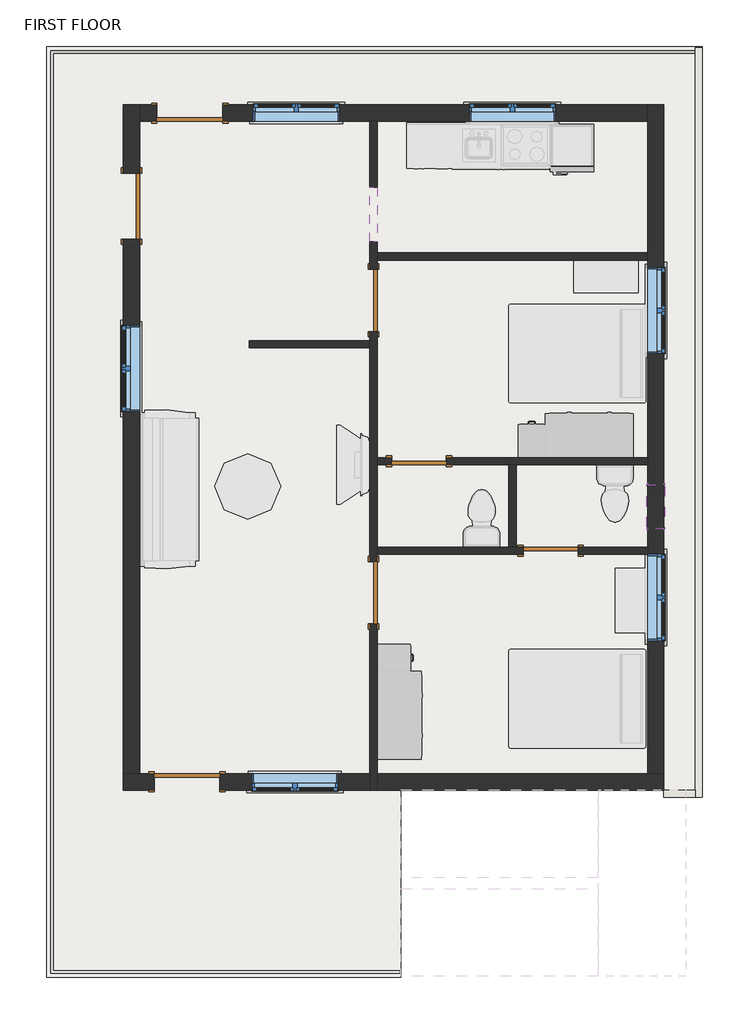
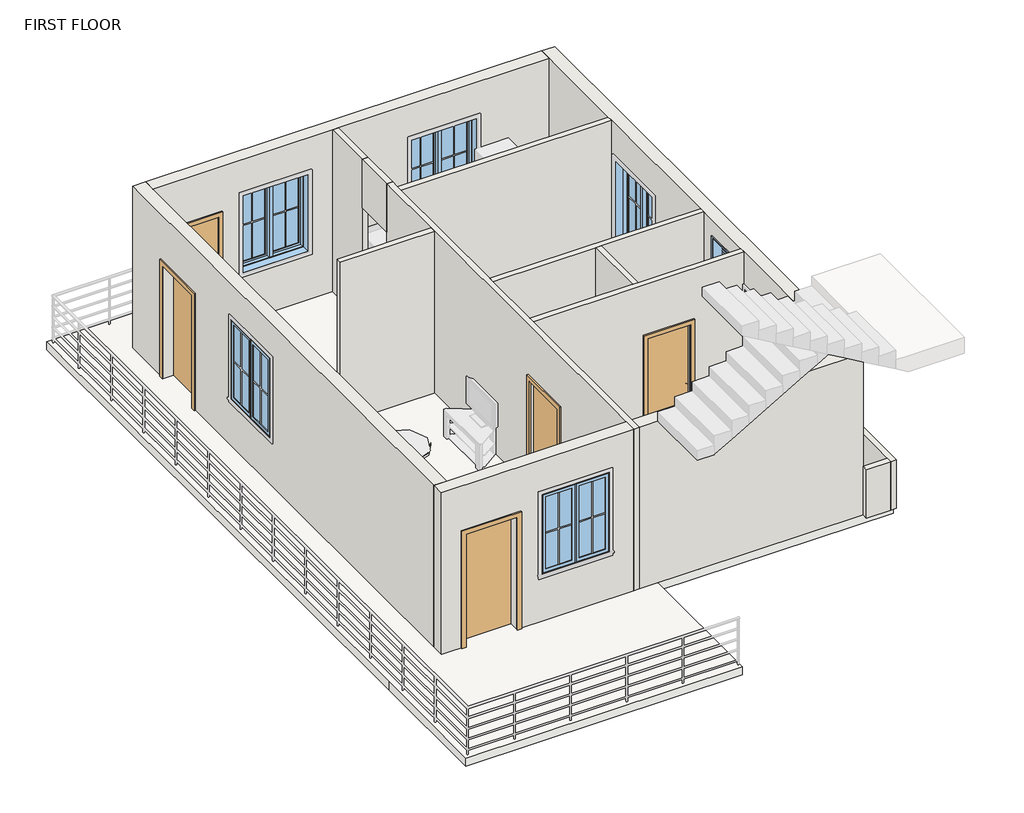
# One storey, part 1 of 3: 15 walls, 7 doors, 7 windows, 1 slab.
"""IFC4 building model written with IfcOpenShell, lengths in millimetres."""

from ifc_helpers import new_model, si_unit, frame, origin, place, context, project, spatial, polyline, outline, extrude, faceted_brep, transform, mapped, element, save
from components import m_single_flush_0762_x_2032mm_63ada305, m_single_flush_0762_x_2032mm_debabc81, m_single_flush_0864_x_2032mm_c62421c0, m_single_flush_0915_x_2134mm_43602619, m_single_flush_0915_x_2134mm_1ddf3370, m_window_casement_double_1200_x_1500mm_04159c99, window_f2d8fef0

model = new_model("IFC4")

# Units and contexts
model_context = context("Model", 3, world=origin())
ifc_project = project(units=[si_unit("LENGTHUNIT", "METRE", prefix="MILLI")], contexts=[model_context])

# Site, building, storey
site = spatial("IfcSite", under=ifc_project)
building = spatial("IfcBuilding", under=site)
storey = spatial("IfcBuildingStorey", under=building, Name="FIRST FLOOR", Elevation=3200.4)

# Doors
placement = place(None, origin())
m_single_flush_0762_x_2032mm_shape = m_single_flush_0762_x_2032mm_63ada305(model_context)
element("IfcDoor", 1, ObjectType="M_Single-Flush : 0762 x 2032mm", at=placement, inside=storey, context=model_context, shape_type="MappedRepresentation", body=[
    mapped(m_single_flush_0762_x_2032mm_shape, transform((2297.1455952, -1088.4648653, 3200.4), x_axis=(-1.0, 0.0, 0.0), y_axis=(0.0, -1.0, 0.0), z_axis=(0.0, 0.0, 1.0))),
])
m_single_flush_0762_x_2032mm_2_shape = m_single_flush_0762_x_2032mm_debabc81(model_context)
element("IfcDoor", 2, ObjectType="M_Single-Flush : 0762 x 2032mm", at=placement, inside=storey, context=model_context, shape_type="MappedRepresentation", body=[
    mapped(m_single_flush_0762_x_2032mm_2_shape, transform((466.7455952, 156.1351347, 3200.4), x_axis=(-1.0, 0.0, 0.0), y_axis=(0.0, -1.0, 0.0), z_axis=(0.0, 0.0, 1.0))),
])
m_single_flush_0864_x_2032mm_shape = m_single_flush_0864_x_2032mm_c62421c0(model_context)
element("IfcDoor", 3, ObjectType="M_Single-Flush : 0864 x 2032mm", at=placement, inside=storey, context=model_context, shape_type="MappedRepresentation", body=[
    mapped(m_single_flush_0864_x_2032mm_shape, transform((-165.0544048, 2391.3351347, 3200.4), x_axis=(0.0, 1.0, 0.0), y_axis=(-1.0, 0.0, 0.0), z_axis=(0.0, 0.0, 1.0))),
])
element("IfcDoor", 4, ObjectType="M_Single-Flush : 0864 x 2032mm", at=placement, inside=storey, context=model_context, shape_type="MappedRepresentation", body=[
    mapped(m_single_flush_0864_x_2032mm_shape, transform((-165.0544048, -1671.2648653, 3200.4), x_axis=(0.0, 1.0, 0.0), y_axis=(-1.0, 0.0, 0.0), z_axis=(0.0, 0.0, 1.0))),
])
m_single_flush_0915_x_2134mm_shape = m_single_flush_0915_x_2134mm_43602619(model_context)
element("IfcDoor", 5, ObjectType="M_Single-Flush : 0915 x 2134mm", at=placement, inside=storey, context=model_context, shape_type="MappedRepresentation", body=[
    mapped(m_single_flush_0915_x_2134mm_shape, transform((-3530.5544048, 3703.0351347, 3200.4), x_axis=(0.0, 1.0, 0.0), y_axis=(-1.0, 0.0, 0.0), z_axis=(0.0, 0.0, 1.0))),
])
element("IfcDoor", 6, ObjectType="M_Single-Flush : 0915 x 2134mm", at=placement, inside=storey, context=model_context, shape_type="MappedRepresentation", body=[
    mapped(m_single_flush_0915_x_2134mm_shape, transform((-2758.7544048, -4301.5648653, 3200.4), x_axis=(-1.0, 0.0, 0.0), y_axis=(0.0, -1.0, 0.0), z_axis=(0.0, 0.0, 1.0))),
])
m_single_flush_0915_x_2134mm_2_shape = m_single_flush_0915_x_2134mm_1ddf3370(model_context)
element("IfcDoor", 7, ObjectType="M_Single-Flush : 0915 x 2134mm", at=placement, inside=storey, context=model_context, shape_type="MappedRepresentation", body=[
    mapped(m_single_flush_0915_x_2134mm_2_shape, transform((-2718.7544048, 4994.8351347, 3200.4), x_axis=(-1.0, 0.0, 0.0), y_axis=(0.0, -1.0, 0.0), z_axis=(0.0, 0.0, 1.0))),
])

# Slab
element("IfcSlab", 8, ObjectType="6\" floor", at=placement, inside=storey, context=model_context, shape_type="SweptSolid", body=[
    extrude(outline(polyline([(4406.9455952, 5921.9351347), (4406.9455952, -4415.8648653), (215.9455952, -4415.8648653), (215.9455952, -7021.8741001), (-4711.6544048, -7021.8741001), (-4711.6544048, -4637.8294487), (-4711.6544048, 5921.9351347), (4406.9455952, 5921.9351347)])), frame((0.0, 0.0, 3048.0), z_axis=(0.0, 0.0, 1.0), x_axis=(1.0, 0.0, 0.0)), (0.0, 0.0, 1.0), 152.4),
])

# Walls
element("IfcWall", 9, ObjectType="4\" wall", at=placement, inside=storey, context=model_context, shape_type="Brep", body=[
    faceted_brep([(-215.8544048, 3204.1351347, 3200.4), (-215.8544048, 2823.3351347, 3200.4), (-215.8544048, 2823.3351347, 5232.4), (-215.8544048, 1959.3351347, 5232.4), (-215.8544048, 1959.3351347, 3200.4), (-215.8544048, 1832.5351347, 3200.4), (-215.8544048, 1730.9351347, 3200.4), (-215.8544048, -1239.2648653, 3200.4), (-215.8544048, -1239.2648653, 5232.4), (-215.8544048, -2103.2648653, 5232.4), (-215.8544048, -2103.2648653, 3200.4), (-215.8544048, -4187.2648653, 3200.4), (-215.8544048, -4415.8648653, 3200.4), (-215.8544048, -4415.8648653, 6248.4), (-215.8544048, -4187.2648653, 6248.4), (-215.8544048, 1730.9351347, 6248.4), (-215.8544048, 1832.5351347, 6248.4), (-215.8544048, 3204.1351347, 6248.4), (-215.8544048, 3204.1351347, 5334.0), (-114.2544048, 2823.3351347, 5232.4), (-114.2544048, 2823.3351347, 3200.4), (-114.2544048, 2950.1351347, 3200.4), (-114.2544048, 3051.7351347, 3200.4), (-114.2544048, 3204.1351347, 3200.4), (-114.2544048, 3204.1351347, 5334.0), (-114.2544048, 3204.1351347, 6248.4), (-114.2544048, 3051.7351347, 6248.4), (-114.2544048, 2950.1351347, 6248.4), (-114.2544048, 206.9351347, 6248.4), (-114.2544048, 105.3351347, 6248.4), (-114.2544048, -1037.6648653, 6248.4), (-114.2544048, -1139.2648653, 6248.4), (-114.2544048, -4187.2648653, 6248.4), (-114.2544048, -4415.8648653, 6248.4), (-114.2544048, -4415.8648653, 3200.4), (-114.2544048, -4187.2648653, 3200.4), (-114.2544048, -2103.2648653, 3200.4), (-114.2544048, -2103.2648653, 5232.4), (-114.2544048, -1239.2648653, 5232.4), (-114.2544048, -1239.2648653, 3200.4), (-114.2544048, -1139.2648653, 3200.4), (-114.2544048, -1037.6648653, 3200.4), (-114.2544048, 105.3351347, 3200.4), (-114.2544048, 206.9351347, 3200.4), (-114.2544048, 1959.3351347, 3200.4), (-114.2544048, 1959.3351347, 5232.4)], [[[0, 1, 2, 3, 4, 5, 6, 7, 8, 9, 10, 11, 12, 13, 14, 15, 16, 17, 18]], [[19, 20, 21, 22, 23, 24, 25, 26, 27, 28, 29, 30, 31, 32, 33, 34, 35, 36, 37, 38, 39, 40, 41, 42, 43, 44, 45]], [[34, 12, 11, 10, 36, 35]], [[23, 22, 21, 20, 1, 0]], [[44, 43, 42, 41, 40, 39, 7, 6, 5, 4]], [[17, 16, 15, 14, 13, 33, 32, 31, 30, 29, 28, 27, 26, 25]], [[0, 18, 17, 25, 24, 23]], [[13, 12, 34, 33]], [[8, 38, 37, 9]], [[9, 37, 36, 10]], [[4, 3, 45, 44]], [[3, 2, 19, 45]], [[2, 1, 20, 19]], [[38, 8, 7, 39]]]),
])
element("IfcWall", 10, ObjectType="4\" wall", at=placement, inside=storey, context=model_context, shape_type="Brep", body=[
    faceted_brep([(-114.2544048, -1139.2648653, 3200.4), (1916.1455952, -1139.2648653, 3200.4), (1916.1455952, -1139.2648653, 5232.4), (2678.1455952, -1139.2648653, 5232.4), (2678.1455952, -1139.2648653, 3200.4), (3644.9455952, -1139.2648653, 3200.4), (3644.9455952, -1139.2648653, 4100.4), (3644.9455952, -1139.2648653, 5600.4), (3644.9455952, -1139.2648653, 6248.4), (-114.2544048, -1139.2648653, 6248.4), (1916.1455952, -1037.6648653, 5232.4), (1916.1455952, -1037.6648653, 3200.4), (1816.1455952, -1037.6648653, 3200.4), (1714.5455952, -1037.6648653, 3200.4), (-114.2544048, -1037.6648653, 3200.4), (-114.2544048, -1037.6648653, 6248.4), (1714.5455952, -1037.6648653, 6248.4), (1816.1455952, -1037.6648653, 6248.4), (3644.9455952, -1037.6648653, 6248.4), (3644.9455952, -1037.6648653, 3200.4), (2678.1455952, -1037.6648653, 3200.4), (2678.1455952, -1037.6648653, 5232.4)], [[[0, 1, 2, 3, 4, 5, 6, 7, 8, 9]], [[10, 11, 12, 13, 14, 15, 16, 17, 18, 19, 20, 21]], [[20, 19, 5, 4]], [[14, 13, 12, 11, 1, 0]], [[9, 8, 18, 17, 16, 15]], [[8, 7, 6, 5, 19, 18]], [[0, 9, 15, 14]], [[2, 1, 11, 10]], [[3, 2, 10, 21]], [[4, 3, 21, 20]]]),
])
element("IfcWall", 11, ObjectType="4\" wall", at=placement, inside=storey, context=model_context, shape_type="Brep", body=[
    faceted_brep([(85.7455952, 206.9351347, 5232.4), (85.7455952, 206.9351347, 3200.4), (-114.2544048, 206.9351347, 3200.4), (-114.2544048, 206.9351347, 6248.4), (3644.9455952, 206.9351347, 6248.4), (3644.9455952, 206.9351347, 3200.4), (847.7455952, 206.9351347, 3200.4), (847.7455952, 206.9351347, 5232.4), (-114.2544048, 105.3351347, 3200.4), (85.7455952, 105.3351347, 3200.4), (85.7455952, 105.3351347, 5232.4), (847.7455952, 105.3351347, 5232.4), (847.7455952, 105.3351347, 3200.4), (1714.5455952, 105.3351347, 3200.4), (1816.1455952, 105.3351347, 3200.4), (3644.9455952, 105.3351347, 3200.4), (3644.9455952, 105.3351347, 6248.4), (1816.1455952, 105.3351347, 6248.4), (1714.5455952, 105.3351347, 6248.4), (-114.2544048, 105.3351347, 6248.4)], [[[0, 1, 2, 3, 4, 5, 6, 7]], [[8, 9, 10, 11, 12, 13, 14, 15, 16, 17, 18, 19]], [[6, 5, 15, 14, 13, 12]], [[2, 1, 9, 8]], [[4, 3, 19, 18, 17, 16]], [[5, 4, 16, 15]], [[3, 2, 8, 19]], [[10, 9, 1, 0]], [[11, 10, 0, 7]], [[12, 11, 7, 6]]]),
])
element("IfcWall", 12, ObjectType="4\" wall", at=placement, inside=storey, context=model_context, shape_type="SweptSolid", body=[
    extrude(outline(polyline([(-215.8544048, 1730.9351347), (-1892.2544048, 1730.9351347), (-1892.2544048, 1832.5351347), (-215.8544048, 1832.5351347), (-215.8544048, 1730.9351347)])), frame((0.0, 0.0, 3200.4), z_axis=(0.0, 0.0, 1.0), x_axis=(1.0, 0.0, 0.0)), (0.0, 0.0, 1.0), 3048.0),
])
element("IfcWall", 13, ObjectType="4\" wall", at=placement, inside=storey, context=model_context, shape_type="SweptSolid", body=[
    extrude(outline(polyline([(-114.2544048, 3051.7351347), (3644.9455952, 3051.7351347), (3644.9455952, 2950.1351347), (-114.2544048, 2950.1351347), (-114.2544048, 3051.7351347)])), frame((0.0, 0.0, 3200.4), z_axis=(0.0, 0.0, 1.0), x_axis=(1.0, 0.0, 0.0)), (0.0, 0.0, 1.0), 3048.0),
])
element("IfcWall", 14, ObjectType="4\" wall", at=placement, inside=storey, context=model_context, shape_type="SweptSolid", body=[
    extrude(outline(polyline([(1714.5455952, -1037.6648653), (1714.5455952, 105.3351347), (1816.1455952, 105.3351347), (1816.1455952, -1037.6648653), (1714.5455952, -1037.6648653)])), frame((0.0, 0.0, 3200.4), z_axis=(0.0, 0.0, 1.0), x_axis=(1.0, 0.0, 0.0)), (0.0, 0.0, 1.0), 3048.0),
])
element("IfcWall", 15, ObjectType="4\" wall", at=placement, inside=storey, context=model_context, shape_type="Brep", body=[
    faceted_brep([(-215.8544048, 4880.5351347, 3200.4), (-215.8544048, 3966.1351347, 3200.4), (-215.8544048, 3966.1351347, 5334.0), (-215.8544048, 3966.1351347, 6248.4), (-215.8544048, 4880.5351347, 6248.4), (-114.2544048, 4880.5351347, 3200.4), (-114.2544048, 4880.5351347, 6248.4), (-114.2544048, 3966.1351347, 6248.4), (-114.2544048, 3966.1351347, 5334.0), (-114.2544048, 3966.1351347, 3200.4)], [[[0, 1, 2, 3, 4]], [[5, 6, 7, 8, 9]], [[1, 0, 5, 9]], [[3, 2, 1, 9, 8, 7]], [[4, 3, 7, 6]], [[0, 4, 6, 5]]]),
])
element("IfcWall", 16, ObjectType="4\" wall", at=placement, inside=storey, context=model_context, shape_type="SweptSolid", body=[
    extrude(outline(polyline([(-215.8544048, 3204.1351347), (-215.8544048, 3966.1351347), (-114.2544048, 3966.1351347), (-114.2544048, 3204.1351347), (-215.8544048, 3204.1351347)])), frame((0.0, 0.0, 5334.0), z_axis=(0.0, 0.0, 1.0), x_axis=(1.0, 0.0, 0.0)), (0.0, 0.0, 1.0), 914.4),
])
element("IfcWall", 17, ObjectType="4\" wall", at=placement, inside=storey, context=model_context, shape_type="Brep", body=[
    faceted_brep([(4305.3455952, 5901.9351347, 3200.4), (4305.3455952, -4415.8648653, 3200.4), (4305.3455952, -4517.4648653, 3200.4), (4305.3455952, -4517.4648653, 4114.8), (4305.3455952, -4415.8648653, 4114.8), (4305.3455952, 5901.9351347, 4114.8), (4406.9455952, 5901.9351347, 3200.4), (4406.9455952, 5901.9351347, 4114.8), (4406.9455952, -4517.4648653, 4114.8), (4406.9455952, -4517.4648653, 3200.4)], [[[0, 1, 2, 3, 4, 5]], [[6, 7, 8, 9]], [[2, 1, 0, 6, 9]], [[5, 4, 3, 8, 7]], [[0, 5, 7, 6]], [[3, 2, 9, 8]]]),
])
element("IfcWall", 18, ObjectType="4\" wall", at=placement, inside=storey, context=model_context, shape_type="SweptSolid", body=[
    extrude(outline(polyline([(3873.5455952, -4415.8648653), (4305.3455952, -4415.8648653), (4305.3455952, -4517.4648653), (3873.5455952, -4517.4648653), (3873.5455952, -4415.8648653)])), frame((0.0, 0.0, 3200.4), z_axis=(0.0, 0.0, 1.0), x_axis=(1.0, 0.0, 0.0)), (0.0, 0.0, 1.0), 914.4),
])
element("IfcWall", 19, ObjectType="9\" wall", at=placement, inside=storey, context=model_context, shape_type="Brep", body=[
    faceted_brep([(-3644.8544048, 5109.1351347, 3200.4), (-3644.8544048, 4160.5351347, 3200.4), (-3644.8544048, 4160.5351347, 5334.4), (-3644.8544048, 3245.5351347, 5334.4), (-3644.8544048, 3245.5351347, 3200.4), (-3644.8544048, -4187.2648653, 3200.4), (-3644.8544048, -4187.2648653, 6248.4), (-3644.8544048, 5109.1351347, 6248.4), (-3644.8544048, 2045.5351347, 5600.4), (-3644.8544048, 845.5351347, 5600.4), (-3644.8544048, 845.5351347, 4100.4), (-3644.8544048, 2045.5351347, 4100.4), (-3416.2544048, 4160.5351347, 5334.4), (-3416.2544048, 4160.5351347, 3200.4), (-3416.2544048, 4880.5351347, 3200.4), (-3416.2544048, 5109.1351347, 3200.4), (-3416.2544048, 5109.1351347, 6248.4), (-3416.2544048, 4880.5351347, 6248.4), (-3416.2544048, -4187.2648653, 6248.4), (-3416.2544048, -4187.2648653, 3200.4), (-3416.2544048, 3245.5351347, 3200.4), (-3416.2544048, 3245.5351347, 5334.4), (-3416.2544048, 2045.5351347, 5600.4), (-3416.2544048, 2045.5351347, 4100.4), (-3416.2544048, 845.5351347, 4100.4), (-3416.2544048, 845.5351347, 5600.4)], [[[0, 1, 2, 3, 4, 5, 6, 7], [8, 9, 10, 11]], [[12, 13, 14, 15, 16, 17, 18, 19, 20, 21], [22, 23, 24, 25]], [[20, 19, 5, 4]], [[15, 14, 13, 1, 0]], [[7, 6, 18, 17, 16]], [[0, 7, 16, 15]], [[2, 1, 13, 12]], [[3, 2, 12, 21]], [[4, 3, 21, 20]], [[23, 22, 8, 11]], [[24, 23, 11, 10]], [[25, 24, 10, 9]], [[22, 25, 9, 8]], [[6, 5, 19, 18]]]),
])
element("IfcWall", 20, ObjectType="9\" wall", at=placement, inside=storey, context=model_context, shape_type="Brep", body=[
    faceted_brep([(-114.2544048, -4415.8648653, 3200.4), (3873.5455952, -4415.8648653, 3200.4), (3873.5455952, -4415.8648653, 6248.4), (-114.2544048, -4415.8648653, 6248.4), (-114.2544048, -4187.2648653, 3200.4), (-114.2544048, -4187.2648653, 6248.4), (3644.9455952, -4187.2648653, 6248.4), (3873.5455952, -4187.2648653, 6248.4), (3873.5455952, -4187.2648653, 3200.4), (3644.9455952, -4187.2648653, 3200.4)], [[[0, 1, 2, 3]], [[4, 5, 6, 7, 8, 9]], [[1, 0, 4, 9, 8]], [[3, 2, 7, 6, 5]], [[0, 3, 5, 4]], [[2, 1, 8, 7]]]),
])
element("IfcWall", 21, ObjectType="9\" wall", at=placement, inside=storey, context=model_context, shape_type="Brep", body=[
    faceted_brep([(3873.5455952, -4187.2648653, 3200.4), (3873.5455952, 5109.1351347, 3200.4), (3873.5455952, 5109.1351347, 6248.4), (3873.5455952, -4187.2648653, 6248.4), (3873.5455952, 1650.1351347, 5600.4), (3873.5455952, 2850.1351347, 5600.4), (3873.5455952, 2850.1351347, 4100.4), (3873.5455952, 1650.1351347, 4100.4), (3873.5455952, -2339.2648653, 5600.4), (3873.5455952, -1139.2648653, 5600.4), (3873.5455952, -1139.2648653, 4100.4), (3873.5455952, -2339.2648653, 4100.4), (3873.5455952, -170.8898653, 5943.6), (3873.5455952, -170.8898653, 5334.0), (3873.5455952, -780.4898653, 5334.0), (3873.5455952, -780.4898653, 5943.6), (3644.9455952, -4187.2648653, 3200.4), (3644.9455952, -4187.2648653, 6248.4), (3644.9455952, -1139.2648653, 6248.4), (3644.9455952, -1037.6648653, 6248.4), (3644.9455952, 105.3351347, 6248.4), (3644.9455952, 206.9351347, 6248.4), (3644.9455952, 2950.1351347, 6248.4), (3644.9455952, 3051.7351347, 6248.4), (3644.9455952, 4880.5351347, 6248.4), (3644.9455952, 5109.1351347, 6248.4), (3644.9455952, 5109.1351347, 3200.4), (3644.9455952, 4880.5351347, 3200.4), (3644.9455952, 3051.7351347, 3200.4), (3644.9455952, 2950.1351347, 3200.4), (3644.9455952, 206.9351347, 3200.4), (3644.9455952, 105.3351347, 3200.4), (3644.9455952, -1037.6648653, 3200.4), (3644.9455952, -1139.2648653, 3200.4), (3644.9455952, 1650.1351347, 5600.4), (3644.9455952, 1650.1351347, 4100.4), (3644.9455952, 2850.1351347, 4100.4), (3644.9455952, 2850.1351347, 5600.4), (3644.9455952, -2339.2648653, 5600.4), (3644.9455952, -2339.2648653, 4100.4), (3644.9455952, -1139.2648653, 4100.4), (3644.9455952, -1139.2648653, 5600.4), (3644.9455952, -170.8898653, 5943.6), (3644.9455952, -780.4898653, 5943.6), (3644.9455952, -780.4898653, 5334.0), (3644.9455952, -170.8898653, 5334.0)], [[[0, 1, 2, 3], [4, 5, 6, 7], [8, 9, 10, 11], [12, 13, 14, 15]], [[16, 17, 18, 19, 20, 21, 22, 23, 24, 25, 26, 27, 28, 29, 30, 31, 32, 33], [34, 35, 36, 37], [38, 39, 40, 41], [42, 43, 44, 45]], [[1, 0, 16, 33, 32, 31, 30, 29, 28, 27, 26]], [[3, 2, 25, 24, 23, 22, 21, 20, 19, 18, 17]], [[0, 3, 17, 16]], [[2, 1, 26, 25]], [[35, 34, 4, 7]], [[36, 35, 7, 6]], [[37, 36, 6, 5]], [[34, 37, 5, 4]], [[39, 38, 8, 11]], [[40, 39, 11, 10]], [[41, 40, 10, 9]], [[38, 41, 9, 8]], [[13, 12, 42, 45]], [[14, 13, 45, 44]], [[15, 14, 44, 43]], [[12, 15, 43, 42]]]),
])
element("IfcWall", 22, ObjectType="9\" wall", at=placement, inside=storey, context=model_context, shape_type="Brep", body=[
    faceted_brep([(-3176.2544048, 5109.1351347, 5334.4), (-3176.2544048, 5109.1351347, 3200.4), (-3416.2544048, 5109.1351347, 3200.4), (-3416.2544048, 5109.1351347, 6248.4), (3644.9455952, 5109.1351347, 6248.4), (3644.9455952, 5109.1351347, 3200.4), (-2261.2544048, 5109.1351347, 3200.4), (-2261.2544048, 5109.1351347, 5334.4), (2365.3455952, 5109.1351347, 5600.4), (1165.3455952, 5109.1351347, 5600.4), (1165.3455952, 5109.1351347, 4100.4), (2365.3455952, 5109.1351347, 4100.4), (-638.5544048, 5109.1351347, 5600.4), (-1838.5544048, 5109.1351347, 5600.4), (-1838.5544048, 5109.1351347, 4100.4), (-638.5544048, 5109.1351347, 4100.4), (-3416.2544048, 4880.5351347, 3200.4), (-3176.2544048, 4880.5351347, 3200.4), (-3176.2544048, 4880.5351347, 5334.4), (-2261.2544048, 4880.5351347, 5334.4), (-2261.2544048, 4880.5351347, 3200.4), (-215.8544048, 4880.5351347, 3200.4), (-114.2544048, 4880.5351347, 3200.4), (3644.9455952, 4880.5351347, 3200.4), (3644.9455952, 4880.5351347, 6248.4), (-114.2544048, 4880.5351347, 6248.4), (-215.8544048, 4880.5351347, 6248.4), (-3416.2544048, 4880.5351347, 6248.4), (2365.3455952, 4880.5351347, 5600.4), (2365.3455952, 4880.5351347, 4100.4), (1165.3455952, 4880.5351347, 4100.4), (1165.3455952, 4880.5351347, 5600.4), (-638.5544048, 4880.5351347, 5600.4), (-638.5544048, 4880.5351347, 4100.4), (-1838.5544048, 4880.5351347, 4100.4), (-1838.5544048, 4880.5351347, 5600.4)], [[[0, 1, 2, 3, 4, 5, 6, 7], [8, 9, 10, 11], [12, 13, 14, 15]], [[16, 17, 18, 19, 20, 21, 22, 23, 24, 25, 26, 27], [28, 29, 30, 31], [32, 33, 34, 35]], [[6, 5, 23, 22, 21, 20]], [[2, 1, 17, 16]], [[4, 3, 27, 26, 25, 24]], [[5, 4, 24, 23]], [[3, 2, 16, 27]], [[18, 17, 1, 0]], [[19, 18, 0, 7]], [[20, 19, 7, 6]], [[29, 28, 8, 11]], [[30, 29, 11, 10]], [[31, 30, 10, 9]], [[28, 31, 9, 8]], [[33, 32, 12, 15]], [[34, 33, 15, 14]], [[35, 34, 14, 13]], [[32, 35, 13, 12]]]),
])
element("IfcWall", 23, ObjectType="9\" wall", at=placement, inside=storey, context=model_context, shape_type="Brep", body=[
    faceted_brep([(-3644.8544048, -4415.8648653, 3200.4), (-3216.2544048, -4415.8648653, 3200.4), (-3216.2544048, -4415.8648653, 5334.4), (-2301.2544048, -4415.8648653, 5334.4), (-2301.2544048, -4415.8648653, 3200.4), (-215.8544048, -4415.8648653, 3200.4), (-215.8544048, -4415.8648653, 6248.4), (-3644.8544048, -4415.8648653, 6248.4), (-1858.5544048, -4415.8648653, 5600.4), (-658.5544048, -4415.8648653, 5600.4), (-658.5544048, -4415.8648653, 4100.4), (-1858.5544048, -4415.8648653, 4100.4), (-3216.2544048, -4187.2648653, 5334.4), (-3216.2544048, -4187.2648653, 3200.4), (-3416.2544048, -4187.2648653, 3200.4), (-3644.8544048, -4187.2648653, 3200.4), (-3644.8544048, -4187.2648653, 6248.4), (-3416.2544048, -4187.2648653, 6248.4), (-215.8544048, -4187.2648653, 6248.4), (-215.8544048, -4187.2648653, 3200.4), (-2301.2544048, -4187.2648653, 3200.4), (-2301.2544048, -4187.2648653, 5334.4), (-1858.5544048, -4187.2648653, 5600.4), (-1858.5544048, -4187.2648653, 4100.4), (-658.5544048, -4187.2648653, 4100.4), (-658.5544048, -4187.2648653, 5600.4)], [[[0, 1, 2, 3, 4, 5, 6, 7], [8, 9, 10, 11]], [[12, 13, 14, 15, 16, 17, 18, 19, 20, 21], [22, 23, 24, 25]], [[20, 19, 5, 4]], [[15, 14, 13, 1, 0]], [[7, 6, 18, 17, 16]], [[2, 1, 13, 12]], [[3, 2, 12, 21]], [[4, 3, 21, 20]], [[23, 22, 8, 11]], [[24, 23, 11, 10]], [[25, 24, 10, 9]], [[22, 25, 9, 8]], [[6, 5, 19, 18]], [[0, 7, 16, 15]]]),
])

# Windows
m_window_casement_double_1200_x_1500mm_shape = m_window_casement_double_1200_x_1500mm_04159c99(model_context)
element("IfcWindow", 24, ObjectType="M_Window-Casement-Double : 1200 x 1500mm", at=placement, inside=storey, context=model_context, shape_type="MappedRepresentation", body=[
    mapped(m_window_casement_double_1200_x_1500mm_shape, transform((1765.3455952, 4994.8351347, 3200.4), x_axis=(1.0, 0.0, 0.0), y_axis=(0.0, 1.0, 0.0), z_axis=(0.0, 0.0, 1.0))),
])
element("IfcWindow", 25, ObjectType="M_Window-Casement-Double : 1200 x 1500mm", at=placement, inside=storey, context=model_context, shape_type="MappedRepresentation", body=[
    mapped(m_window_casement_double_1200_x_1500mm_shape, transform((3759.2455952, 2250.1351347, 3200.4), x_axis=(0.0, -1.0, 0.0), y_axis=(1.0, 0.0, 0.0), z_axis=(0.0, 0.0, 1.0))),
])
element("IfcWindow", 26, ObjectType="M_Window-Casement-Double : 1200 x 1500mm", at=placement, inside=storey, context=model_context, shape_type="MappedRepresentation", body=[
    mapped(m_window_casement_double_1200_x_1500mm_shape, transform((3759.2455952, -1739.2648653, 3200.4), x_axis=(0.0, -1.0, 0.0), y_axis=(1.0, 0.0, 0.0), z_axis=(0.0, 0.0, 1.0))),
])
element("IfcWindow", 27, ObjectType="M_Window-Casement-Double : 1200 x 1500mm", at=placement, inside=storey, context=model_context, shape_type="MappedRepresentation", body=[
    mapped(m_window_casement_double_1200_x_1500mm_shape, transform((-3530.5544048, 1445.5351347, 3200.4), x_axis=(0.0, 1.0, 0.0), y_axis=(-1.0, 0.0, 0.0), z_axis=(0.0, 0.0, 1.0))),
])
element("IfcWindow", 28, ObjectType="M_Window-Casement-Double : 1200 x 1500mm", at=placement, inside=storey, context=model_context, shape_type="MappedRepresentation", body=[
    mapped(m_window_casement_double_1200_x_1500mm_shape, transform((-1238.5544048, 4994.8351347, 3200.4), x_axis=(1.0, 0.0, 0.0), y_axis=(0.0, 1.0, 0.0), z_axis=(0.0, 0.0, 1.0))),
])
element("IfcWindow", 29, ObjectType="M_Window-Casement-Double : 1200 x 1500mm", at=placement, inside=storey, context=model_context, shape_type="MappedRepresentation", body=[
    mapped(m_window_casement_double_1200_x_1500mm_shape, transform((-1258.5544048, -4301.5648653, 3200.4), x_axis=(-1.0, 0.0, 0.0), y_axis=(0.0, -1.0, 0.0), z_axis=(0.0, 0.0, 1.0))),
])
window_shape = window_f2d8fef0(model_context)
element("IfcWindow", 30, ObjectType="Window-Louvers : 24\" x 24\"", at=placement, inside=storey, context=model_context, shape_type="MappedRepresentation", body=[
    mapped(window_shape, transform((3765.5955952, -475.6898653, 4419.6), x_axis=(0.0, -1.0, 0.0), y_axis=(1.0, 0.0, 0.0), z_axis=(0.0, 0.0, 1.0))),
])

save(model, "model.ifc")

# Revit data of these elements
# Type "M_Single-Flush : 0762 x 2032mm"
#   Type Mark = "28"
#   Construction Type Id = "MDOOR"
#   Analytic Construction = "Metal"
#   Thickness = 0.167323 ft
#   Thermal Resistance (R) = 0.270117 (m²·K)/W
#   Heat Transfer Coefficient (U) = 3.7021 W/(m²·K)
#   Height = 6.666667 ft
#   Trim Projection Ext = 0.082021 ft
#   Trim Projection Int = 0.082021 ft
#   Trim Width = 0.249344 ft
#   Width = 2.5 ft
#   Define Thermal Properties by = 1
#   Define Thermal Properties by = 1
#   Door Material = Door - Panel
#   Frame Material = Door - Frame
#   Visual Light Transmittance = 0
#   Solar Heat Gain Coefficient = 0
#   Function = (empty or 0)
#   Wall Closure = (empty or 0)
# Type "M_Single-Flush : 0864 x 2032mm"
#   Type Mark = "32"
#   Construction Type Id = "MDOOR"
#   Analytic Construction = "Metal"
#   Thickness = 0.167323 ft
#   Thermal Resistance (R) = 0.270117 (m²·K)/W
#   Heat Transfer Coefficient (U) = 3.7021 W/(m²·K)
#   Height = 6.666667 ft
#   Trim Projection Ext = 0.082021 ft
#   Trim Projection Int = 0.082021 ft
#   Trim Width = 0.249344 ft
#   Width = 2.834646 ft
#   Define Thermal Properties by = 1
#   Define Thermal Properties by = 1
#   Door Material = Door - Panel
#   Frame Material = Door - Frame
#   Visual Light Transmittance = 0
#   Solar Heat Gain Coefficient = 0
#   Function = (empty or 0)
#   Wall Closure = (empty or 0)
# Type "M_Single-Flush : 0915 x 2134mm"
#   Type Mark = "20"
#   Construction Type Id = "MDOOR"
#   Analytic Construction = "Metal"
#   Thickness = 0.167323 ft
#   Thermal Resistance (R) = 0.270117 (m²·K)/W
#   Heat Transfer Coefficient (U) = 3.7021 W/(m²·K)
#   Height = 7.001312 ft
#   Trim Projection Ext = 0.082021 ft
#   Trim Projection Int = 0.082021 ft
#   Trim Width = 0.249344 ft
#   Width = 3.001969 ft
#   Define Thermal Properties by = 1
#   Define Thermal Properties by = 1
#   Door Material = Door - Panel
#   Frame Material = Door - Frame
#   Visual Light Transmittance = 0
#   Solar Heat Gain Coefficient = 0
#   Function = (empty or 0)
#   Wall Closure = (empty or 0)
# Type "6\" floor"
#   Function = 0
#   Layers, outside or top first: 0.5 ft no material (function 1)
# Type "4\" wall"
#   Layers, outside or top first: 0.333333 ft no material (function 1)
# Type "9\" wall"
#   Layers, outside or top first: 0.75 ft no material (function 1)
# Type "M_Window-Casement-Double : 1200 x 1500mm"
#   Type Mark = "25"
#   Fire Rating = "0.5h"
#   Assembly Code = "B2020100"
#   Analytic Construction = "Double glazing - domestic"
#   Frame Extension [instance default] = 0.020833 ft
#   Window Inset [instance default] = 0.0 ft
#   Wall Thickness [instance default] = 0.492126 ft
#   Interior Wall Closure [instance default] = 0.179626 ft
#   Half Width = 1.968504 ft
#   Visual Light Transmittance = 0.81
#   Thermal Resistance (R) = 0.319569 (m²·K)/W
#   Solar Heat Gain Coefficient = 0.76
#   Rough Width = 3.98622 ft
#   Rough Height = 4.970472 ft
#   Height = 4.92126 ft
#   Heat Transfer Coefficient (U) = 3.12929 W/(m²·K)
#   Exterior Wall Closure [instance default] = 0.104331 ft
#   Extension Jamb [instance default] = 0.179626 ft
#   Default Sill Height = 2.952756 ft
#   Width = 3.937008 ft
#   Define Thermal Properties by = 0
#   Muntin Visibility = yes
#   Interior Trim Visibility [instance default] = yes
#   Exterior Trim Visibility [instance default] = yes
#   Extension Jamb Visibility [instance default] = yes
#   Interior Trim Material = Wood - Stained
#   Muntin Pattern = M_Muntin Pattern_2x2 : M_Muntin Pattern_2x2
#   Interior Trim = M_Trim-Window-Interior-Flat : Picture Frame
#   Interior Frame Material = Wood - Stained
#   Glass Panel Material = Glass
#   Exterior Trim Material = Clad - White
#   Exterior Trim = M_Trim-Window-Exterior-Flat : with Sill
#   Exterior Frame Material = Clad - White
#   Wall Closure = (empty or 0)
# Type "Window-Louvers : 24\" x 24\""
#   Type Mark = "28"
#   Construction Type Id = "GSP4R"
#   Assembly Code = "B20"
#   Analytic Construction = "1/8 in Pilkington single glazing"
#   Visual Light Transmittance = 0.9
#   Thermal Resistance (R) = 0.271106 (m²·K)/W
#   Solar Heat Gain Coefficient = 0.78
#   Max Height = 1.978553 ft
#   Height = 2.0 ft
#   Heat Transfer Coefficient (U) = 3.6886 W/(m²·K)
#   Blade Width [instance default] = 1.875 ft
#   Blade Vertical Thickness = 0.029463 ft
#   Blade Thickness = 0.020833 ft
#   Blade Spacing = 0.125 ft
#   Blade Height = 0.154463 ft
#   Blade Depth = 0.25 ft
#   Blade Angle = 45.00°
#   Default Sill Height = 3.0 ft
#   Trim Projection_Exterior = 0.041667 ft
#   Trim Projection_Interior = 0.041667 ft
#   Trim Width_Exterior = 0.125 ft
#   Trim Width_Interior = 0.125 ft
#   Width = 2.0 ft
#   Max Blade Count = 12
#   Define Thermal Properties by = 1
#   Blade Count = 12
#   Frame Material = Birch
#   Louver Material = Birch
#   Trim Exterior Material = Birch
#   Trim Interior Material = Birch
#   Wall Closure = (empty or 0)
# Elements 1, 2 (IfcDoor, "M_Single-Flush : 0762 x 2032mm")
#   Phase Created = New Construction
#   Materials on its faces: "Door - Frame", "Door - Panel"
# Elements 3, 4 (IfcDoor, "M_Single-Flush : 0864 x 2032mm")
#   Phase Created = New Construction
#   Materials on its faces: "Door - Frame", "Door - Panel"
# Elements 5, 6, 7 (IfcDoor, "M_Single-Flush : 0915 x 2134mm")
#   Phase Created = New Construction
#   Materials on its faces: "Door - Frame", "Door - Panel"
# Element 8 (IfcSlab, "6\" floor")
#   Height Offset From Level = 0.0 ft
#   Phase Created = New Construction
#   Materials on its faces: "Default Floor"
# Elements 9, 10, 11, 12, 13, 14, 15 (IfcWall, "4\" wall")
#   Top Offset = 0.0 ft
#   Base Offset = 0.0 ft
#   Unconnected Height = 10.0 ft
#   wall height = 10.0 ft
#   Phase Created = New Construction
#   Base Constraint = FIRST FLOOR
#   Materials on its faces: "Default Wall"
# Element 16 (IfcWall, "4\" wall")
#   built-in parameter 1001111 = 7.0 ft
#   Top Offset = 0.0 ft
#   Base Offset = 7.0 ft
#   Unconnected Height = 3.0 ft
#   wall height = 3.0 ft
#   Phase Created = New Construction
#   Base Constraint = FIRST FLOOR
#   Materials on its faces: "Default Wall"
# Elements 17, 18 (IfcWall, "4\" wall")
#   Top Offset = 0.0 ft
#   Base Offset = 0.0 ft
#   Unconnected Height = 3.0 ft
#   wall height = 3.0 ft
#   Phase Created = New Construction
#   Base Constraint = FIRST FLOOR
#   Materials on its faces: "Default Wall"
# Elements 19, 20, 21, 22, 23 (IfcWall, "9\" wall")
#   Top Offset = 0.0 ft
#   Base Offset = 0.0 ft
#   Unconnected Height = 10.0 ft
#   wall height = 10.0 ft
#   Phase Created = New Construction
#   Base Constraint = FIRST FLOOR
#   Materials on its faces: "Default Wall"
# Element 24 (IfcWindow, "M_Window-Casement-Double : 1200 x 1500mm")
#   Mark = "8"
#   Window Inset = 0.0 ft
#   Interior Wall Closure = 0.179626 ft
#   Frame Extension = 0.020833 ft
#   Exterior Wall Closure = 0.104331 ft
#   Interior Trim Visibility = yes
#   Exterior Trim Visibility = yes
#   Phase Created = New Construction
#   Materials on its faces: "Wood - Stained", "Glass", "Clad - White"
# Element 25 (IfcWindow, "M_Window-Casement-Double : 1200 x 1500mm")
#   Mark = "9"
#   Window Inset = 0.0 ft
#   Interior Wall Closure = 0.179626 ft
#   Frame Extension = 0.020833 ft
#   Exterior Wall Closure = 0.104331 ft
#   Interior Trim Visibility = yes
#   Exterior Trim Visibility = yes
#   Phase Created = New Construction
#   Materials on its faces: "Wood - Stained", "Glass", "Clad - White"
# Element 26 (IfcWindow, "M_Window-Casement-Double : 1200 x 1500mm")
#   Mark = "10"
#   Window Inset = 0.0 ft
#   Interior Wall Closure = 0.179626 ft
#   Frame Extension = 0.020833 ft
#   Exterior Wall Closure = 0.104331 ft
#   Interior Trim Visibility = yes
#   Exterior Trim Visibility = yes
#   Phase Created = New Construction
#   Materials on its faces: "Wood - Stained", "Glass", "Clad - White"
# Element 27 (IfcWindow, "M_Window-Casement-Double : 1200 x 1500mm")
#   Mark = "12"
#   Window Inset = 0.0 ft
#   Interior Wall Closure = 0.179626 ft
#   Frame Extension = 0.020833 ft
#   Exterior Wall Closure = 0.104331 ft
#   Interior Trim Visibility = yes
#   Exterior Trim Visibility = yes
#   Phase Created = New Construction
#   Materials on its faces: "Wood - Stained", "Glass", "Clad - White"
# Element 28 (IfcWindow, "M_Window-Casement-Double : 1200 x 1500mm")
#   Mark = "13"
#   Window Inset = 0.0 ft
#   Interior Wall Closure = 0.179626 ft
#   Frame Extension = 0.020833 ft
#   Exterior Wall Closure = 0.104331 ft
#   Interior Trim Visibility = yes
#   Exterior Trim Visibility = yes
#   Phase Created = New Construction
#   Materials on its faces: "Wood - Stained", "Glass", "Clad - White"
# Element 29 (IfcWindow, "M_Window-Casement-Double : 1200 x 1500mm")
#   Mark = "22"
#   Window Inset = 0.0 ft
#   Interior Wall Closure = 0.179626 ft
#   Frame Extension = 0.020833 ft
#   Exterior Wall Closure = 0.104331 ft
#   Interior Trim Visibility = yes
#   Exterior Trim Visibility = yes
#   Phase Created = New Construction
#   Materials on its faces: "Wood - Stained", "Glass", "Clad - White"
# Element 30 (IfcWindow, "Window-Louvers : 24\" x 24\"")
#   Mark = "14"
#   Blade Width = 1.875 ft
#   Phase Created = New Construction
#   Materials on its faces: "Birch"
# Materials
#   "Door - Panel": class "Wood", colour RGB 210 159 95, transparency 0, Cost = 0
#   "Door - Frame": colour RGB 118 70 51, transparency 0, Cost = 0
#   "Wood - Stained": class "Wood", colour RGB 224 178 126, transparency 0, Cost = 0
#   "Glass": class "Glass", colour RGB 0 128 192, transparency 0.9, Description = "Soda Lime Glass", Cost = 0
#   "Clad - White": class "Wood", colour RGB 242 242 238, transparency 0, Cost = 0
#   "Birch": class "Wood", colour RGB 224 178 126, transparency 0, Description = "Betula Alleghaniensis", Cost = 0
#   "Default Floor": colour RGB 127 127 127, transparency 0, Cost = 0
#   "Default Wall": colour RGB 128 128 128, transparency 0, Cost = 0
